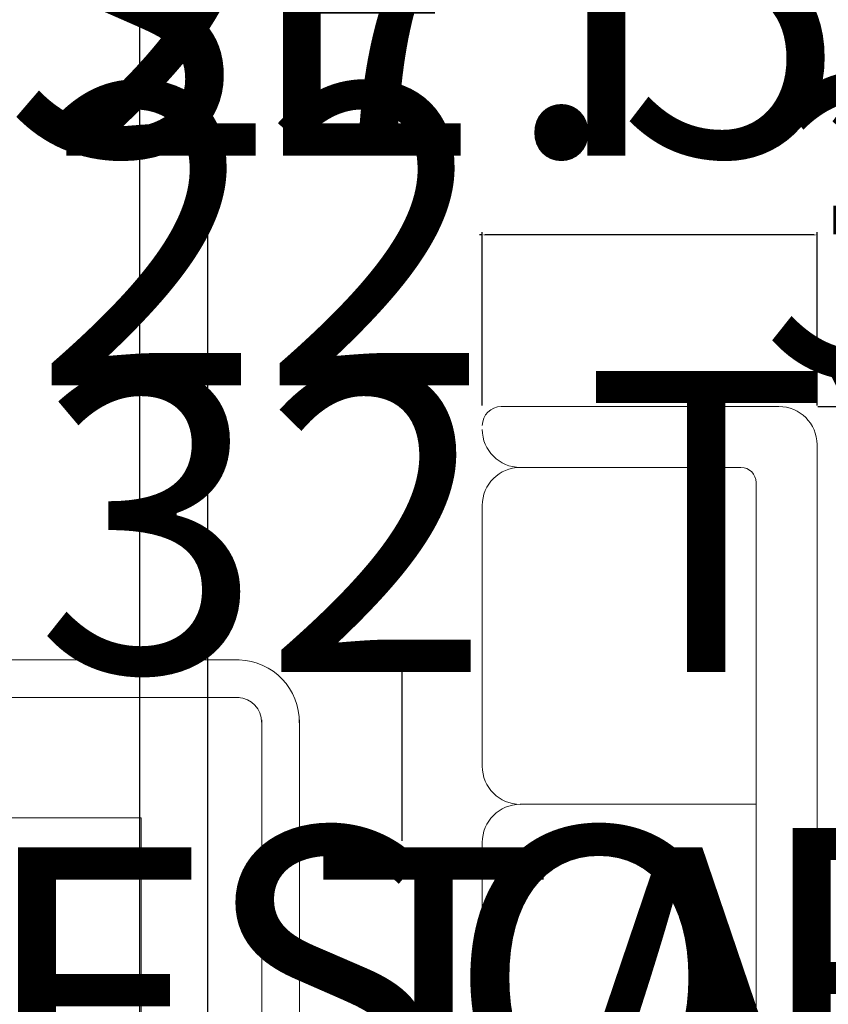
# Model space of a CAD drawing. Units: inches. Extents: x 305 to 776, y 38 to 479.
# Tile 10 of 14: x 458 to 511, y 214 to 280. Entities that reach past the tile are written whole.
import ezdxf

# ---------------------------------------------------------------- set-up
doc = ezdxf.new("R2010")
doc.units = ezdxf.units.IN
doc.header["$MEASUREMENT"] = 0
doc.layers.add('A-ANNO-DIMS', color=2, linetype='Continuous', lineweight=18)
doc.layers.add('A-FURN', color=8, linetype='Continuous', lineweight=18)
doc.styles.get("Standard").update_dxf_attribs({"font": 'arial.ttf'})
doc.dimstyles.get("Standard").update_dxf_attribs({"dimtxt": 20, "dimasz": 0.18, "dimexe": 0.18, "dimexo": 0.0625, "dimgap": 0.09, "dimtad": 0, "dimtih": 1, "dimtoh": 1, "dimdec": 4, "dimzin": 0, "dimdsep": 46, "dimtxsty": 'Standard', "dimcen": 0.09, "dimadec": 0, "dimazin": 0, "dimtfac": 1, "dimtdec": 4, "dimtofl": 0, "dimtmove": 0, "dimatfit": 3, "dimfxl": 1, "dimtolj": 1, "dimtzin": 0, "dimarcsym": 0})

# ---------------------------------------------------------------- blocks, each defined once
blk = doc.blocks.new('sofa-25')
at = {"color": 0, "linetype": 'ByBlock'}
for p, q in [((1.0702, 0.5197), (0.6532, 0.5197)), ((1.5935, 0.5197), (1.1883, 0.5197)), ((1.7471, 0.0591), (1.7471, 0.4902)), ((1.1293, 0.0945), (1.1293, 0.4607)), ((1.6526, 0.1181), (1.6526, 0.4607)), ((0.0945, 0.0945), (1.6289, 0.0945)), ((0, 0), (1.688, 0))]:
    blk.add_line(p, q, dxfattribs=at)
for centre, radius, start, end in [((1.0702, 0.4607), 0.0591, 0, 90), ((1.1883, 0.4607), 0.0591, 90, 180), ((1.5935, 0.4607), 0.0591, 0, 90), ((1.7116, 0.4607), 0.0591, 90, 180), ((1.7175, 0.4902), 0.0295, 0, 90), ((1.6289, 0.1181), 0.0236, 270, 0), ((1.688, 0.0591), 0.0591, 270, 0)]:
    blk.add_arc(centre, radius, start, end, dxfattribs=at)
blk = doc.blocks.new('carp')
for p, q in [((853.971, 318.32), (853.971, 318.33)), ((857.971, 314.33), (857.965, 314.33))]:
    blk.add_line(p, q)
for points in [[(853.971, 318.33), (831.574, 318.33)], [(853.971, 315.83), (831.574, 315.83)], [(827.971, 314.727), (827.971, 277.33)], [(830.471, 314.727), (830.471, 277.33)], [(855.471, 277.33), (855.471, 314.33)], [(857.971, 277.33), (857.971, 314.33)], [(831.971, 275.83), (853.971, 275.83)], [(831.971, 273.33), (853.971, 273.33)]]:
    blk.add_lwpolyline(points)
blk.add_lwpolyline([(838.471, 307.83), (838.471, 283.83), (847.471, 283.83), (847.471, 307.83)], close=True)
for centre, radius, start, end in [((831.772, 314.528), 3.807, 87.01121, 182.98879), ((853.855, 314.211), 4.111, 358.88612, 88.46258), ((831.772, 314.528), 1.307, 87.01121, 182.98879), ((853.855, 314.211), 1.611, 358.88612, 88.46258), ((832.523, 277.882), 2.086, 186.91602, 263.08398), ((853.419, 277.882), 2.086, 276.91602, 353.08398), ((832.523, 277.882), 4.586, 186.91602, 263.08398), ((853.419, 277.882), 4.586, 276.91602, 353.08398)]:
    blk.add_arc(centre, radius, start, end)
blk = doc.blocks.new('*D19')
at = {"layer": 'A-ANNO-DIMS', "color": 0, "lineweight": -2, "transparency": 16777216}
for p, q in [((557.633, 250.82), (557.633, 245.977)), ((589.133, 250.82), (589.133, 245.977)), ((557.633, 246.157), (557.453, 246.157)), ((588.953, 246.157), (557.813, 246.157))]:
    blk.add_line(p, q, dxfattribs=at)
at = {"layer": 'A-ANNO-DIMS', "color": 0, "transparency": 16777216}
for points in [[(557.813, 246.187), (557.813, 246.127), (557.633, 246.157)], [(588.953, 246.187), (588.953, 246.127), (589.133, 246.157)]]:
    blk.add_solid(points, dxfattribs=at)
at = {"layer": 'Defpoints', "color": 0, "transparency": 16777216}
for p in [(557.633, 250.882), (589.133, 250.882), (557.633, 246.157)]:
    blk.add_point(p, dxfattribs=at)
at = {"layer": 'A-ANNO-DIMS', "color": 0, "transparency": 16777216, "insert": (463.393, 246.157), "char_height": 20, "attachment_point": 5}
blk.add_mtext('\\A1;DOOR 32 TYP.', dxfattribs=at)
blk = doc.blocks.new('*D20')
at = {"layer": 'A-ANNO-DIMS', "color": 0, "lineweight": -2, "transparency": 16777216}
for p, q in [((557.57, 280.724), (552.728, 280.724)), ((552.908, 280.544), (552.908, 276.111)), ((552.908, 251.062), (552.908, 255.495)), ((557.57, 250.882), (552.728, 250.882))]:
    blk.add_line(p, q, dxfattribs=at)
at = {"layer": 'A-ANNO-DIMS', "color": 0, "transparency": 16777216}
for points in [[(552.878, 280.544), (552.938, 280.544), (552.908, 280.724)], [(552.878, 251.062), (552.938, 251.062), (552.908, 250.882)]]:
    blk.add_solid(points, dxfattribs=at)
at = {"layer": 'Defpoints', "color": 0, "transparency": 16777216}
for p in [(552.908, 280.724), (557.633, 280.724), (557.633, 250.882)]:
    blk.add_point(p, dxfattribs=at)
at = {"layer": 'A-ANNO-DIMS', "color": 0, "transparency": 16777216, "insert": (552.908, 265.803), "char_height": 20, "attachment_point": 5}
blk.add_mtext('\\A1;30 TYP.', dxfattribs=at)
blk = doc.blocks.new('*D33')
at = {"layer": 'A-ANNO-DIMS', "color": 0, "lineweight": -2, "transparency": 16777216}
for p, q in [((440.927, 307.949), (449.29, 307.949)), ((449.11, 307.769), (449.11, 290.896)), ((449.11, 253.161), (449.11, 270.034)), ((440.927, 252.981), (449.29, 252.981))]:
    blk.add_line(p, q, dxfattribs=at)
at = {"layer": 'A-ANNO-DIMS', "color": 0, "transparency": 16777216}
for points in [[(449.08, 307.769), (449.14, 307.769), (449.11, 307.949)], [(449.08, 253.161), (449.14, 253.161), (449.11, 252.981)]]:
    blk.add_solid(points, dxfattribs=at)
at = {"layer": 'Defpoints', "color": 0, "transparency": 16777216}
for p in [(440.864, 307.949), (449.11, 307.949), (440.864, 252.981)]:
    blk.add_point(p, dxfattribs=at)
at = {"layer": 'A-ANNO-DIMS', "color": 0, "transparency": 16777216, "insert": (449.11, 280.465), "char_height": 20, "attachment_point": 5}
blk.add_mtext('\\A1;DINING SET 55', dxfattribs=at)
blk = doc.blocks.new('*D35')
at = {"layer": 'A-ANNO-DIMS', "color": 0, "lineweight": -2, "transparency": 16777216}
for p, q in [((510.695, 253.802), (522.215, 253.802)), ((522.035, 253.622), (522.035, 226.234)), ((522.035, 177.97), (522.035, 205.358)), ((510.695, 177.79), (522.215, 177.79))]:
    blk.add_line(p, q, dxfattribs=at)
at = {"layer": 'A-ANNO-DIMS', "color": 0, "transparency": 16777216}
for points in [[(522.005, 253.622), (522.065, 253.622), (522.035, 253.802)], [(522.005, 177.97), (522.065, 177.97), (522.035, 177.79)]]:
    blk.add_solid(points, dxfattribs=at)
at = {"layer": 'Defpoints', "color": 0, "transparency": 16777216}
for p in [(510.633, 253.802), (522.035, 253.802), (510.633, 177.79)]:
    blk.add_point(p, dxfattribs=at)
at = {"layer": 'A-ANNO-DIMS', "color": 0, "transparency": 16777216, "insert": (522.035, 215.796), "char_height": 20, "attachment_point": 5}
blk.add_mtext('\\A1;SOFA 76', dxfattribs=at)
blk = doc.blocks.new('*D36')
at = {"layer": 'A-ANNO-DIMS', "color": 0, "lineweight": -2, "transparency": 16777216}
for p, q in [((488.396, 265.203), (488.216, 265.203)), ((488.396, 253.864), (488.396, 265.383)), ((510.453, 265.203), (488.576, 265.203)), ((510.633, 253.864), (510.633, 265.383))]:
    blk.add_line(p, q, dxfattribs=at)
at = {"layer": 'A-ANNO-DIMS', "color": 0, "transparency": 16777216}
for points in [[(488.576, 265.233), (488.576, 265.173), (488.396, 265.203)], [(510.453, 265.233), (510.453, 265.173), (510.633, 265.203)]]:
    blk.add_solid(points, dxfattribs=at)
at = {"layer": 'Defpoints', "color": 0, "transparency": 16777216}
for p in [(488.396, 265.203), (488.396, 253.802), (510.633, 253.802)]:
    blk.add_point(p, dxfattribs=at)
at = {"layer": 'A-ANNO-DIMS', "color": 0, "transparency": 16777216, "insert": (473.733, 265.203), "char_height": 20, "attachment_point": 5}
blk.add_mtext('\\A1;22', dxfattribs=at)
blk = doc.blocks.new('*D37')
at = {"layer": 'A-ANNO-DIMS', "color": 0, "lineweight": -2, "transparency": 16777216}
for p, q in [((476.346, 237.029), (483.222, 237.029)), ((483.042, 236.849), (483.042, 224.939)), ((483.042, 192.153), (483.042, 204.063)), ((476.346, 191.973), (483.222, 191.973))]:
    blk.add_line(p, q, dxfattribs=at)
at = {"layer": 'A-ANNO-DIMS', "color": 0, "transparency": 16777216}
for points in [[(483.012, 236.849), (483.072, 236.849), (483.042, 237.029)], [(483.012, 192.153), (483.072, 192.153), (483.042, 191.973)]]:
    blk.add_solid(points, dxfattribs=at)
at = {"layer": 'Defpoints', "color": 0, "transparency": 16777216}
for p in [(476.283, 237.029), (483.042, 237.029), (476.283, 191.973)]:
    blk.add_point(p, dxfattribs=at)
at = {"layer": 'A-ANNO-DIMS', "color": 0, "transparency": 16777216, "insert": (483.042, 214.501), "char_height": 20, "attachment_point": 5}
blk.add_mtext('\\A1;COFFEE TABLE 45', dxfattribs=at)
blk = doc.blocks.new('*D47')
at = {"layer": 'A-ANNO-DIMS', "color": 0, "lineweight": -2, "transparency": 16777216}
for p, q in [((465.633, 331.82), (465.633, 51.201)), ((470.133, 331.82), (470.133, 51.201)), ((465.813, 51.381), (469.953, 51.381)), ((470.133, 51.381), (470.313, 51.381))]:
    blk.add_line(p, q, dxfattribs=at)
at = {"layer": 'A-ANNO-DIMS', "color": 0, "transparency": 16777216}
for points in [[(465.813, 51.411), (465.813, 51.351), (465.633, 51.381)], [(469.953, 51.411), (469.953, 51.351), (470.133, 51.381)]]:
    blk.add_solid(points, dxfattribs=at)
at = {"layer": 'Defpoints', "color": 0, "transparency": 16777216}
for p in [(465.633, 331.882), (470.133, 331.882), (470.133, 51.381)]:
    blk.add_point(p, dxfattribs=at)
at = {"layer": 'A-ANNO-DIMS', "color": 0, "transparency": 16777216, "insert": (489.086, 51.381), "char_height": 20, "attachment_point": 5}
blk.add_mtext('\\A1;4.5', dxfattribs=at)
blk = doc.blocks.new('*D60')
at = {"layer": 'A-ANNO-DIMS', "color": 0, "lineweight": -2, "transparency": 16777216}
for p, q in [((428.263, 331.82), (428.263, 51.201)), ((465.633, 331.82), (465.633, 51.201)), ((428.443, 51.381), (465.453, 51.381)), ((465.633, 51.381), (465.813, 51.381))]:
    blk.add_line(p, q, dxfattribs=at)
at = {"layer": 'A-ANNO-DIMS', "color": 0, "transparency": 16777216}
for points in [[(428.443, 51.411), (428.443, 51.351), (428.263, 51.381)], [(465.453, 51.411), (465.453, 51.351), (465.633, 51.381)]]:
    blk.add_solid(points, dxfattribs=at)
at = {"layer": 'Defpoints', "color": 0, "transparency": 16777216}
for p in [(428.263, 331.882), (465.633, 331.882), (465.633, 51.381)]:
    blk.add_point(p, dxfattribs=at)
at = {"layer": 'A-ANNO-DIMS', "color": 0, "transparency": 16777216, "insert": (499.641, 51.381), "char_height": 20, "attachment_point": 5}
blk.add_mtext('\\A1;37.37', dxfattribs=at)
blk = doc.blocks.new('*D61')
at = {"layer": 'A-ANNO-DIMS', "color": 0, "lineweight": -2, "transparency": 16777216}
for p, q in [((437.73, 398.686), (437.73, 51.201)), ((465.633, 398.686), (465.633, 51.201)), ((437.91, 51.381), (465.453, 51.381)), ((465.633, 51.381), (465.813, 51.381))]:
    blk.add_line(p, q, dxfattribs=at)
at = {"layer": 'A-ANNO-DIMS', "color": 0, "transparency": 16777216}
for points in [[(437.91, 51.411), (437.91, 51.351), (437.73, 51.381)], [(465.453, 51.411), (465.453, 51.351), (465.633, 51.381)]]:
    blk.add_solid(points, dxfattribs=at)
at = {"layer": 'Defpoints', "color": 0, "transparency": 16777216}
for p in [(437.73, 398.749), (465.633, 398.749), (465.633, 51.381)]:
    blk.add_point(p, dxfattribs=at)
at = {"layer": 'A-ANNO-DIMS', "color": 0, "transparency": 16777216, "insert": (492.069, 51.381), "char_height": 20, "attachment_point": 5}
blk.add_mtext('\\A1;27.9', dxfattribs=at)
blk = doc.blocks.new('*D62')
at = {"layer": 'A-ANNO-DIMS', "color": 0, "lineweight": -2, "transparency": 16777216}
for p, q in [((399.633, 336.32), (399.633, 51.201)), ((423.233, 336.32), (423.233, 51.201)), ((399.813, 51.381), (423.053, 51.381)), ((423.233, 51.381), (423.413, 51.381))]:
    blk.add_line(p, q, dxfattribs=at)
at = {"layer": 'A-ANNO-DIMS', "color": 0, "transparency": 16777216}
for points in [[(399.813, 51.411), (399.813, 51.351), (399.633, 51.381)], [(423.053, 51.411), (423.053, 51.351), (423.233, 51.381)]]:
    blk.add_solid(points, dxfattribs=at)
at = {"layer": 'Defpoints', "color": 0, "transparency": 16777216}
for p in [(399.633, 336.382), (423.233, 336.382), (423.233, 51.381)]:
    blk.add_point(p, dxfattribs=at)
at = {"layer": 'A-ANNO-DIMS', "color": 0, "transparency": 16777216, "insert": (449.642, 51.381), "char_height": 20, "attachment_point": 5}
blk.add_mtext('\\A1;23.6', dxfattribs=at)
blk = doc.blocks.new('*D65')
at = {"layer": 'A-ANNO-DIMS', "color": 0, "lineweight": -2, "transparency": 16777216}
for p, q in [((399.633, 351.219), (399.633, 51.201)), ((421.89, 351.219), (421.89, 51.201)), ((399.813, 51.381), (421.71, 51.381)), ((421.89, 51.381), (422.07, 51.381))]:
    blk.add_line(p, q, dxfattribs=at)
at = {"layer": 'A-ANNO-DIMS', "color": 0, "transparency": 16777216}
for points in [[(399.813, 51.411), (399.813, 51.351), (399.633, 51.381)], [(421.71, 51.411), (421.71, 51.351), (421.89, 51.381)]]:
    blk.add_solid(points, dxfattribs=at)
at = {"layer": 'Defpoints', "color": 0, "transparency": 16777216}
for p in [(399.633, 351.281), (421.89, 351.281), (421.89, 51.381)]:
    blk.add_point(p, dxfattribs=at)
at = {"layer": 'A-ANNO-DIMS', "color": 0, "transparency": 16777216, "insert": (463.844, 51.381), "char_height": 20, "attachment_point": 5}
blk.add_mtext('\\A1;22.257', dxfattribs=at)
blk = doc.blocks.new('*D75')
at = {"layer": 'A-ANNO-DIMS', "color": 0, "lineweight": -2, "transparency": 16777216}
for p, q in [((413.291, 280.465), (413.471, 280.465)), ((413.381, 280.375), (413.381, 280.555)), ((435.396, 280.465), (427.32, 280.465))]:
    blk.add_line(p, q, dxfattribs=at)
at = {"layer": 'A-ANNO-DIMS', "color": 0, "transparency": 16777216}
blk.add_solid([(427.32, 280.495), (427.32, 280.435), (427.14, 280.465)], dxfattribs=at)
at = {"layer": 'Defpoints', "color": 0, "transparency": 16777216}
for p in [(399.621, 280.466), (427.14, 280.465)]:
    blk.add_point(p, dxfattribs=at)
at = {"layer": 'A-ANNO-DIMS', "color": 0, "transparency": 16777216, "insert": (480.009, 280.465), "char_height": 20, "attachment_point": 5}
blk.add_mtext('\\A1;∅27.52', dxfattribs=at)

msp = doc.modelspace()

# ---------------------------------------------------------------- block references
at = {"layer": 'A-FURN', "xscale": 42.78470327655635, "yscale": 42.78470327655635, "zscale": 42.78470327655635, "rotation": 89.99999999999996}
msp.add_blockref('sofa-25', (510.6329, 179.0538), dxfattribs=at)
at = {"layer": 'A-FURN'}
msp.add_blockref('carp', (-381.7264, -81.357), dxfattribs=at)

# ---------------------------------------------------------------- dimensions: what is measured, and where the dimension line sits
at = {"layer": 'A-ANNO-DIMS'}
for base, p1, p2, override, picture, middle in [((465.6329, 51.3805), (437.7303, 398.7487), (465.6329, 398.7487), {"dimdec": 1, "dimlfac": 1, "dimrnd": 0, "dimzin": 0, "dimdsep": 46, "dimlunit": 2}, '*D61', (492.0693, 51.3805)), ((421.8895, 51.3805), (399.6329, 351.2815), (421.8895, 351.2815), {"dimdec": 3, "dimlfac": 1, "dimrnd": 0, "dimzin": 0, "dimdsep": 46, "dimlunit": 2}, '*D65', (463.8444, 51.3805)), ((423.2329, 51.3805), (399.6329, 336.382), (423.2329, 336.382), {"dimdec": 1, "dimlfac": 1, "dimrnd": 0, "dimzin": 0, "dimdsep": 46, "dimlunit": 2}, '*D62', (449.6421, 51.3805)), ((465.6329, 51.3805), (428.2629, 331.882), (465.6329, 331.882), {"dimdec": 2, "dimlfac": 1, "dimrnd": 0, "dimzin": 0, "dimdsep": 46, "dimlunit": 2}, '*D60', (499.641, 51.3805)), ((470.1329, 51.3805), (465.6329, 331.882), (470.1329, 331.882), {"dimdec": 1, "dimlfac": 1, "dimrnd": 0, "dimzin": 0, "dimdsep": 46, "dimlunit": 2}, '*D47', (489.0864, 51.3805))]:
    dim = msp.add_linear_dim(base=base, p1=p1, p2=p2, dimstyle='Standard', override=override, dxfattribs=at)
    dim.commit()
    dim.dimension.update_dxf_attribs({"geometry": picture, "text_midpoint": middle})
for base, p1, p2, angle, text, picture, middle in [((449.1096, 307.9493), (440.8644, 252.9815), (440.8644, 307.9493), 90, 'DINING SET <>', '*D33', (449.1096, 280.4654)), ((552.9079, 280.7241), (557.6329, 250.882), (557.6329, 280.7241), 90, '<> TYP.', '*D20', (552.9079, 265.8031)), ((557.6329062952, 246.15704135), (589.1329062952, 250.88204135), (557.6329062952, 250.88204135), 180, 'DOOR <> TYP.', '*D19', (463.3929199378, 246.15704135)), ((483.0416, 237.0288), (476.2832, 191.9726), (476.2832, 237.0288), 90, 'COFFEE TABLE <>', '*D37', (483.0416, 214.5007)), ((522.0346, 253.8016), (510.6329, 177.7903), (510.6329, 253.8016), 90, 'SOFA <>', '*D35', (522.0346, 215.796))]:
    dim = msp.add_linear_dim(base=base, p1=p1, p2=p2, angle=angle, text=text, dimstyle='Standard', override={"dimdec": 0, "dimlfac": 1, "dimrnd": 0, "dimzin": 0, "dimdsep": 46, "dimlunit": 2}, dxfattribs=at)
    dim.commit()
    dim.dimension.update_dxf_attribs({"geometry": picture, "text_midpoint": middle})
dim = msp.add_diameter_dim_2p(p1=(399.6205, 280.4658), p2=(427.1405, 280.465), dimstyle='Standard', override={"dimdec": 2, "dimlfac": 1, "dimrnd": 0, "dimzin": 0, "dimdsep": 46, "dimlunit": 2}, dxfattribs=at)
dim.commit()
dim.dimension.update_dxf_attribs({"geometry": '*D75', "text_midpoint": (435.3965, 280.4648), "dimtype": 163})
dim = msp.add_linear_dim(base=(488.3956, 265.2033), p1=(510.6329, 253.8016), p2=(488.3956, 253.8016), angle=180, dimstyle='Standard', override={"dimdec": 0, "dimlfac": 1, "dimrnd": 0, "dimzin": 0, "dimdsep": 46, "dimlunit": 2}, dxfattribs=at)
dim.commit()
dim.dimension.update_dxf_attribs({"geometry": '*D36', "text_midpoint": (473.7327, 265.2033)})

doc.saveas('drawing.dxf')
